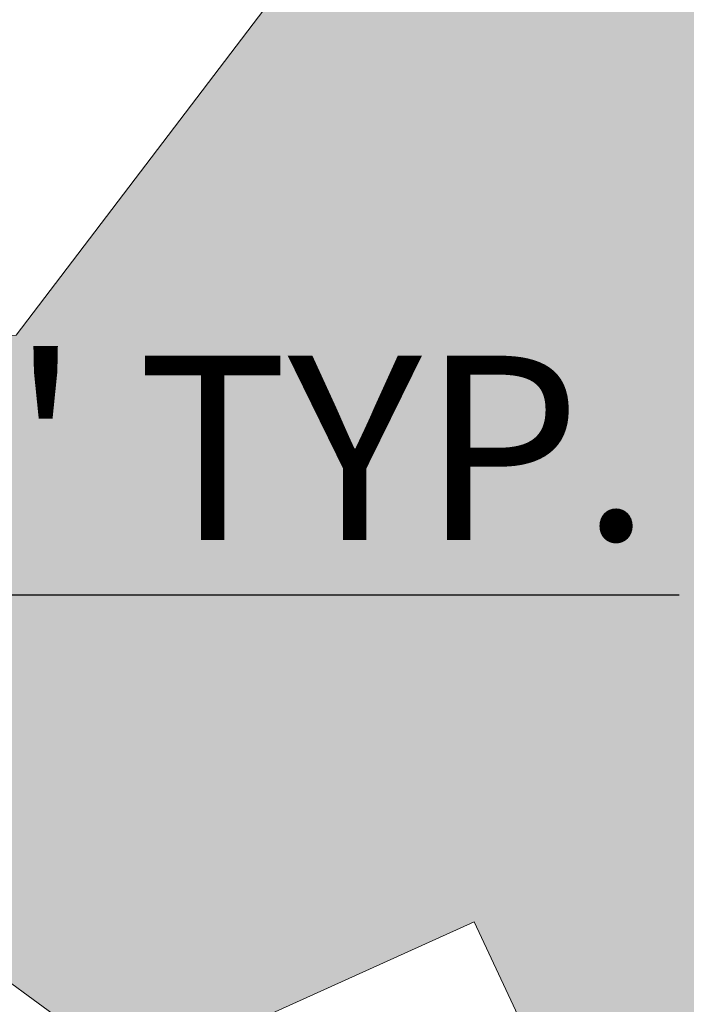
# Model space of a CAD drawing. Units: inches. Extents: x 2091 to 2899, y 967 to 2217.
# Tile 254 of 256: x 2232 to 2246, y 1131 to 1153. Entities that reach past the tile are written whole.
import ezdxf

# ---------------------------------------------------------------- set-up
doc = ezdxf.new("R2010")
doc.units = ezdxf.units.IN
doc.layers.add('A-ANNO-DIMS', color=2, linetype='Continuous', lineweight=18)
doc.layers.add('L-PLNT-TREE', color=94, linetype='Continuous', lineweight=13)
doc.layers.add('A-WALL-PATT', color=141, linetype='Continuous', lineweight=13, true_color=0xadddf7)
doc.layers.add('L-PLNT-PATT', color=114, linetype='Continuous', lineweight=13, true_color=0x139b48)
doc.styles.get("Standard").update_dxf_attribs({"font": 'arial.ttf'})
doc.dimstyles.new('ISO-25', dxfattribs={"dimtxt": 4, "dimasz": 4, "dimexe": 1.25, "dimexo": 0.625, "dimtad": 1, "dimdec": 0, "dimlunit": 3, "dimtxsty": 'Standard', "dimcen": 2.5, "dimadec": 0, "dimazin": 0, "dimtfac": 1, "dimtdec": 0, "dimtmove": 0, "dimatfit": 3, "dimfxl": 1, "dimarcsym": 0})

# ---------------------------------------------------------------- blocks, each defined once
blk = doc.blocks.new('*U25')
blk.add_lwpolyline([(-1139.42368, 1783.79628), (-1216.11644, 1685.47796), (-1117.5111, 1601.2033), (-1051.7759, 1643.3419), (-1126.09884, 1521.20092), (-1072.10606, 1527.49758), (-1079.90386, 1416.93646), (-1259.93906, 1179.83508), (-1479.05978, 1165.78888), (-1577.66258, 1109.60662), (-1742.00312, 927.01364), (-1676.26538, 814.64658), (-1270.89408, 828.69278), (-1194.20386, 772.51052), (-1007.95074, 856.78518), (-876.4778, 575.87134), (-821.70016, 575.87134), (-569.71184, 884.87504)])
blk = doc.blocks.new('*D37')
at = {"layer": 'A-ANNO-DIMS', "color": 0, "lineweight": -2, "transparency": 16777216}
for p, q in [((2203.116, 1151.622), (2203.116, 1138.874)), ((2212.276, 1151.622), (2212.276, 1138.874)), ((2199.116, 1140.124), (2195.116, 1140.124)), ((2203.116, 1140.124), (2212.276, 1140.124)), ((2216.276, 1140.124), (2245.908, 1140.124))]:
    blk.add_line(p, q, dxfattribs=at)
at = {"layer": 'A-ANNO-DIMS', "color": 0, "transparency": 16777216}
for points in [[(2199.116, 1140.79), (2199.116, 1139.457), (2203.116, 1140.124)], [(2216.276, 1140.79), (2216.276, 1139.457), (2212.276, 1140.124)]]:
    blk.add_solid(points, dxfattribs=at)
at = {"layer": 'Defpoints', "color": 0, "transparency": 16777216}
for p in [(2203.116, 1152.247), (2212.276, 1152.247), (2212.276, 1140.124)]:
    blk.add_point(p, dxfattribs=at)
at = {"layer": 'A-ANNO-DIMS', "color": 0, "transparency": 16777216, "insert": (2233.092, 1142.791), "char_height": 4, "attachment_point": 5}
blk.add_mtext('0\'-9" TYP.', dxfattribs=at)
blk = doc.blocks.new('*D71')
at = {"layer": 'A-ANNO-DIMS', "color": 0, "lineweight": -2, "transparency": 16777216}
for p, q in [((2212.144, 1351.294), (2212.144, 969.464)), ((2452.144, 1351.294), (2452.144, 969.464)), ((2216.144, 970.714), (2448.144, 970.714))]:
    blk.add_line(p, q, dxfattribs=at)
at = {"layer": 'A-ANNO-DIMS', "color": 0, "transparency": 16777216}
for points in [[(2216.144, 971.381), (2216.144, 970.048), (2212.144, 970.714)], [(2448.144, 971.381), (2448.144, 970.048), (2452.144, 970.714)]]:
    blk.add_solid(points, dxfattribs=at)
at = {"layer": 'Defpoints', "color": 0, "transparency": 16777216}
for p in [(2212.144, 1351.919), (2452.144, 1351.919), (2452.144, 970.714)]:
    blk.add_point(p, dxfattribs=at)
at = {"layer": 'A-ANNO-DIMS', "color": 0, "transparency": 16777216, "insert": (2332.144, 973.382), "char_height": 4, "attachment_point": 5}
blk.add_mtext('20\'-0"', dxfattribs=at)

msp = doc.modelspace()

# ---------------------------------------------------------------- hatches: boundary and pattern name
at = {"layer": 'A-WALL-PATT'}
h = msp.add_hatch(color=256, dxfattribs=at)
h.dxf.hatch_style = 1
h.paths.add_polyline_path([(2803.144, 2050.919), (2203.144, 2050.919), (2203.144, 1090.919), (2803.144, 1090.919)])
h.paths.add_polyline_path([(2635.799, 1147.54), (2674.524, 1147.54, 0.376086), (2678.53, 1152.88), (2678.53, 1159.556, 0.333335), (2674.524, 1163.562), (2674.524, 1163.562), (2674.524, 1192.934), (2635.806, 1192.934), (2597.088, 1192.934), (2597.088, 1163.562, 0.333335), (2593.082, 1159.556), (2593.082, 1152.88, 0.376086), (2597.088, 1147.54)], flags=0)
h.paths.add_polyline_path([(2436.01, 1278.241, 0.000483), (2435.953, 1278.215, -0.001328), (2435.936, 1278.112, -0.001711), (2436.116, 1278.041, 0.002185)], flags=0)
h.paths.add_polyline_path([(2794.144, 1143.419), (2794.144, 1347.419), (2543.37, 1347.419), (2543.37, 1351.919), (2794.144, 1351.919), (2794.144, 1392.714), (2793.947, 1392.714), (2793.947, 1473.537), (2794.144, 1473.537), (2794.144, 1531.919), (2650.144, 1531.919), (2650.144, 1536.419), (2794.144, 1536.419), (2794.144, 1692.419), (2609.376, 1692.419), (2609.376, 1644.419), (2604.876, 1644.419), (2604.876, 1744.919), (2609.376, 1744.919), (2609.376, 1696.919), (2794.144, 1696.919), (2794.144, 1780.919), (2609.644, 1780.919), (2493.876, 1780.919), (2493.876, 1785.419), (2609.644, 1785.419), (2794.144, 1785.419), (2794.144, 1847.939), (2793.951, 1847.939), (2793.951, 1928.762), (2794.144, 1928.762), (2794.144, 1941.419), (2614.144, 1941.419), (2614.144, 1821.419), (2609.644, 1821.419), (2609.644, 1941.419), (2392.144, 1941.419), (2392.144, 1819.919), (2387.644, 1819.919), (2387.644, 1941.419), (2212.144, 1941.419), (2212.144, 1783.919), (2392.144, 1783.919), (2392.144, 1780.919), (2212.144, 1780.919), (2212.144, 1629.419), (2387.644, 1629.419), (2387.644, 1744.919), (2392.144, 1744.919), (2392.144, 1627.919), (2317.144, 1627.919), (2317.144, 1551.419), (2317.144, 1536.419), (2459.384, 1536.419), (2459.384, 1602.396), (2463.884, 1602.396), (2463.884, 1531.919), (2456.644, 1531.919), (2456.644, 1529.919), (2452.144, 1529.919), (2452.144, 1531.919), (2312.644, 1531.919), (2312.644, 1551.419), (2306.144, 1551.419), (2306.144, 1555.919), (2308.144, 1555.919), (2308.144, 1551.419), (2312.644, 1551.419), (2312.644, 1627.919), (2212.144, 1627.919), (2212.144, 1555.919), (2270.144, 1555.919), (2270.144, 1551.419), (2212.144, 1551.419), (2212.144, 1351.919), (2272.144, 1351.919), (2272.144, 1347.419), (2212.144, 1347.419), (2212.144, 1275.419), (2308.144, 1275.419), (2308.144, 1351.919), (2452.144, 1351.919), (2452.144, 1493.919), (2456.644, 1493.919), (2456.644, 1347.419), (2312.644, 1347.419), (2312.644, 1270.919), (2212.144, 1270.919), (2212.144, 1099.919), (2281.238, 1099.919), (2282.871, 1110.914), (2282.008, 1116.997), (2278.558, 1121.42), (2268.206, 1128.056), (2272.088, 1128.056), (2273.813, 1131.927), (2279.42, 1134.692), (2285.028, 1135.245), (2287.616, 1137.457), (2288.047, 1138.01), (2289.341, 1140.775), (2291.067, 1139.669), (2292.361, 1135.245), (2295.38, 1136.904), (2296.243, 1135.798), (2297.105, 1133.033), (2300.125, 1138.01), (2303.144, 1138.01), (2304.438, 1135.798), (2303.144, 1133.586), (2306.595, 1134.692), (2307.889, 1133.033), (2310.908, 1135.245), (2313.927, 1134.139), (2315.627, 1132.427), (2308.32, 1117.55), (2290.204, 1109.808), (2288.91, 1103.172), (2289.272, 1099.919), (2434.918, 1099.919), (2431.593, 1124.788), (2429.93, 1169.553), (2430.927, 1240.52), (2435.659, 1238.186), (2437.135, 1196.554), (2438.798, 1143.973), (2442.678, 1111.998), (2446.558, 1099.919), (2794.144, 1099.919), (2794.144, 1138.919), (2548.032, 1138.919), (2548.032, 1143.419), (2548.032, 1148.819), (2546.668, 1148.032), (2528.686, 1179.179, 0.256256), (2512.032, 1148.819), (2512.032, 1143.419), (2512.032, 1138.919), (2507.532, 1138.919), (2507.532, 1143.419), (2507.532, 1148.819, 0.256256), (2490.879, 1179.179), (2472.896, 1148.032), (2471.532, 1148.819), (2471.532, 1143.419), (2467.032, 1143.419), (2467.032, 1269.946, 0.039061), (2460.91, 1273.58), (2467.032, 1273.58), (2467.032, 1286.325, 0.014511), (2465.216, 1286.762), (2467.032, 1287.053), (2467.032, 1323.419), (2471.532, 1323.419), (2471.532, 1148.819), (2489.532, 1179.996), (2490.896, 1179.208), (2490.879, 1179.179, -0.256256), (2507.532, 1148.819), (2507.532, 1143.419), (2512.032, 1143.419), (2512.032, 1148.819, -0.256256), (2528.686, 1179.179), (2528.668, 1179.208), (2530.032, 1179.996), (2548.032, 1148.819), (2548.032, 1143.419)], flags=16)
h.paths.add_polyline_path([(2607.769, 1200.945), (2607.769, 1265.031), (2597.088, 1281.052), (2619.785, 1281.052), (2627.795, 1337.127), (2635.799, 1337.127), (2643.817, 1337.127), (2651.827, 1281.052), (2674.524, 1281.052), (2663.843, 1265.031), (2663.843, 1200.945), (2635.806, 1200.945)], flags=0)
edge = h.paths.add_edge_path(flags=0)
edge.add_ellipse((13303.896, 1272.999), major_axis=(-10595.313, 0), ratio=0.84230387, start_angle=0.6282372, end_angle=0.6465541, ccw=False)
edge.add_ellipse((2711.7, 1156.853), major_axis=(2.22, 0), ratio=0.842304, start_angle=111.5352, end_angle=180.6282, ccw=False)
edge.add_ellipse((13303.156, 1272.999), major_axis=(-10593.026, 0), ratio=0.84230387, start_angle=0.5282715, end_angle=0.6465541, ccw=False)
edge.add_line((2710.765, 1175.333), (2710.13, 1175.333))
edge.add_ellipse((2710.13, 1176.58), major_axis=(1.48, 0), ratio=0.842304, start_angle=180, end_angle=270, ccw=False)
edge.add_line((2708.65, 1176.58), (2708.65, 1200.783))
edge.add_ellipse((2710.13, 1200.783), major_axis=(1.48, 0), ratio=0.842304, start_angle=90, end_angle=180, ccw=False)
edge.add_line((2710.13, 1202.029), (2710.465, 1202.029))
edge.add_ellipse((13303.156, 1272.999), major_axis=(-10593.026, 0), ratio=0.84230387, start_angle=-0.0902291, end_angle=0.3838668, ccw=False)
edge.add_ellipse((2710.13, 1290.927), major_axis=(-1.48, 0), ratio=0.842304, start_angle=0, end_angle=90, ccw=False)
edge.add_line((2708.65, 1290.927), (2708.65, 1315.13))
edge.add_ellipse((2710.13, 1315.13), major_axis=(-1.48, 0), ratio=0.842304, start_angle=-90, end_angle=0, ccw=False)
edge.add_line((2710.13, 1316.377), (2710.706, 1316.377))
edge.add_ellipse((3238.402, 1296.29), major_axis=(528.234, 0), ratio=0.8423039, start_angle=176.34957, end_angle=177.82005, ccw=False)
edge.add_ellipse((2775.063, 1071.451), major_axis=(313.308, 0), ratio=0.8423039, start_angle=102.12597, end_angle=103.78053, ccw=False)
edge.add_ellipse((2775.063, 1078.306), major_axis=(-305.303, 0), ratio=0.8423039, start_angle=-79.79046, end_angle=-77.55537, ccw=False)
edge.add_ellipse((2695.142, 1541.975), major_axis=(-250.96, 0), ratio=0.8423039, start_angle=99.25657, end_angle=102.55493)
edge.add_line((2741.41, 1334.214), (2747.133, 1337.378))
edge.add_ellipse((2747.539, 1336.857), major_axis=(-0.74, 0), ratio=0.842304, start_angle=270, end_angle=307.9331, ccw=False)
edge.add_ellipse((2747.539, 1336.857), major_axis=(-0.74, 0), ratio=0.842304, start_angle=232.0669, end_angle=270, ccw=False)
edge.add_line((2747.945, 1337.378), (2753.667, 1334.214))
edge.add_ellipse((2799.935, 1541.975), major_axis=(250.96, 0), ratio=0.8423039, start_angle=257.44507, end_angle=260.74343)
edge.add_ellipse((2720.014, 1078.306), major_axis=(305.303, 0), ratio=0.8423039, start_angle=77.55537, end_angle=79.79046, ccw=False)
edge.add_ellipse((2720.014, 1071.451), major_axis=(-313.308, 0), ratio=0.8423039, start_angle=256.21947, end_angle=257.87403, ccw=False)
edge.add_ellipse((2256.676, 1296.29), major_axis=(-528.234, 0), ratio=0.8423039, start_angle=182.17995, end_angle=183.65043, ccw=False)
edge.add_line((2784.371, 1316.377), (2784.947, 1316.377))
edge.add_ellipse((2784.947, 1315.13), major_axis=(1.48, 0), ratio=0.842304, start_angle=0, end_angle=90, ccw=False)
edge.add_line((2786.427, 1315.13), (2786.427, 1290.927))
edge.add_ellipse((2784.947, 1290.927), major_axis=(1.48, 0), ratio=0.842304, start_angle=270, end_angle=360, ccw=False)
edge.add_ellipse((-7808.079, 1272.999), major_axis=(10593.026, 0), ratio=0.84230387, start_angle=-0.3838668, end_angle=0.0902291, ccw=False)
edge.add_line((2784.612, 1202.029), (2784.947, 1202.029))
edge.add_ellipse((2784.947, 1200.783), major_axis=(1.48, 0), ratio=0.842304, start_angle=0, end_angle=90, ccw=False)
edge.add_line((2786.427, 1200.783), (2786.427, 1176.58))
edge.add_ellipse((2784.947, 1176.58), major_axis=(-1.48, 0), ratio=0.842304, start_angle=90, end_angle=180, ccw=False)
edge.add_line((2784.947, 1175.333), (2784.313, 1175.333))
edge.add_ellipse((-7808.079, 1272.999), major_axis=(10593.026, 0), ratio=0.84230387, start_angle=-0.6186432, end_angle=-0.5282715, ccw=False)
edge.add_ellipse((2783.377, 1156.853), major_axis=(-2.22, 0), ratio=0.842304, start_angle=179.3718, end_angle=248.4648, ccw=False)
edge.add_ellipse((-7808.819, 1272.999), major_axis=(-10595.313, 0), ratio=0.842303866, start_angle=179.3534459, end_angle=179.3717628, ccw=False)
edge.add_ellipse((2780.297, 1153.501), major_axis=(-5.246, 0), ratio=0.842304, start_angle=90, end_angle=179.3534, ccw=False)
edge.add_line((2780.297, 1149.082), (2714.78, 1149.082))
edge.add_ellipse((2714.78, 1153.501), major_axis=(5.246, 0), ratio=0.842304, start_angle=180.6466, end_angle=270, ccw=False)
edge = h.paths.add_edge_path(flags=0)
edge.add_line((2718.187, 1151.008), (2718.187, 1170.472))
edge.add_ellipse((2721.147, 1170.472), major_axis=(-2.96, 0), ratio=0.842304, start_angle=-90, end_angle=0, ccw=False)
edge.add_line((2721.147, 1172.965), (2773.93, 1172.965))
edge.add_ellipse((2773.93, 1170.472), major_axis=(-2.96, 0), ratio=0.842304, start_angle=180, end_angle=270, ccw=False)
edge.add_line((2776.89, 1170.472), (2776.89, 1151.008))
edge.add_line((2776.89, 1151.008), (2718.187, 1151.008))
edge = h.paths.add_edge_path(flags=0)
edge.add_line((2718.187, 1180.234), (2718.187, 1199.058))
edge.add_ellipse((2747.539, 1320.399), major_axis=(147.018, 0), ratio=0.8423039, start_angle=256.40187, end_angle=283.59813)
edge.add_line((2776.89, 1199.058), (2776.89, 1180.234))
edge.add_ellipse((2747.539, 1301.575), major_axis=(147.018, 0), ratio=0.8423039, start_angle=256.40187, end_angle=283.59813, ccw=False)
edge = h.paths.add_edge_path(flags=0)
edge.add_ellipse((13303.156, 1272.999), major_axis=(-10591.546, 0), ratio=0.84230387, start_angle=0.0555943, end_angle=0.3777642, ccw=False)
edge.add_line((2711.617, 1262.722), (2715.667, 1249.495))
edge.add_ellipse((6413.892, 1241.692), major_axis=(-3698.236, 0), ratio=0.84230387, start_angle=-0.120897, end_angle=0.364076)
edge.add_line((2715.761, 1218.192), (2711.934, 1203.167))
edge = h.paths.add_edge_path(flags=0)
edge.add_line((2718.187, 1251.075), (2716.002, 1267.45))
edge.add_ellipse((2742.151, 1202.19), major_axis=(81.773, 0), ratio=0.842304, start_angle=94.27742, end_angle=111.83495, ccw=False)
edge.add_line((2737.01, 1270.931), (2758.067, 1270.931))
edge.add_ellipse((2752.926, 1202.19), major_axis=(81.773, 0), ratio=0.842304, start_angle=68.16505, end_angle=85.72258, ccw=False)
edge.add_line((2779.075, 1267.45), (2776.89, 1251.075))
edge.add_ellipse((2750.338, 1187.885), major_axis=(79.58, 0), ratio=0.842304, start_angle=67.20809, end_angle=85.12993)
edge.add_line((2756.035, 1254.744), (2739.043, 1254.744))
edge.add_ellipse((2744.739, 1187.885), major_axis=(79.58, 0), ratio=0.842304, start_angle=94.87007, end_angle=112.79191)
edge = h.paths.add_edge_path(flags=0)
edge.add_line((2783.143, 1203.167), (2779.316, 1218.192))
edge.add_ellipse((-918.815, 1241.692), major_axis=(3698.236, 0), ratio=0.84230387, start_angle=-0.364076, end_angle=0.120897)
edge.add_line((2779.41, 1249.495), (2783.46, 1262.722))
edge.add_ellipse((-7808.079, 1272.999), major_axis=(-10591.546, 0), ratio=0.84230387, start_angle=179.6222358, end_angle=179.9444057, ccw=False)
edge = h.paths.add_edge_path(flags=0)
edge.add_ellipse((2734.201, 1286.69), major_axis=(-0.357, 6.34), ratio=0.603834, start_angle=89.002, end_angle=253.6574, ccw=False)
edge.add_line((2730.369, 1286.542), (2730.369, 1301.352))
edge.add_line((2730.369, 1301.352), (2735.913, 1305.215))
edge.add_ellipse((2736.385, 1304.735), major_axis=(0.74, 0), ratio=0.842304, start_angle=90, end_angle=134.4802, ccw=False)
edge.add_line((2736.385, 1305.358), (2738.033, 1305.358))
edge.add_line((2738.033, 1305.358), (2738.033, 1307.708))
edge.add_ellipse((2794.202, 1307.708), major_axis=(56.169, 0), ratio=0.842304, start_angle=150.5614, end_angle=180, ccw=False)
edge.add_ellipse((2700.876, 1307.708), major_axis=(-56.169, 0), ratio=0.842304, start_angle=180, end_angle=209.4386, ccw=False)
edge.add_line((2757.044, 1307.708), (2757.044, 1305.358))
edge.add_line((2757.044, 1305.358), (2758.692, 1305.358))
edge.add_ellipse((2758.692, 1304.735), major_axis=(-0.74, 0), ratio=0.842304, start_angle=225.5198, end_angle=270, ccw=False)
edge.add_line((2759.164, 1305.215), (2764.708, 1301.352))
edge.add_line((2764.708, 1301.352), (2764.708, 1286.542))
edge.add_ellipse((2760.876, 1286.69), major_axis=(0.357, 6.34), ratio=0.603834, start_angle=106.3426, end_angle=270.998, ccw=False)
edge.add_line((2757.044, 1285.797), (2757.044, 1307.708))
edge.add_ellipse((2700.876, 1307.708), major_axis=(-56.169, 0), ratio=0.842304, start_angle=180, end_angle=209.4386)
edge.add_ellipse((2794.202, 1307.708), major_axis=(56.169, 0), ratio=0.842304, start_angle=150.5614, end_angle=180)
edge.add_line((2738.033, 1307.708), (2738.033, 1285.797))
h.paths.add_polyline_path([(2417.812, 1104.45), (2413.492, 1102.53), (2410.612, 1103.97), (2409.172, 1106.37), (2407.252, 1107.33), (2406.292, 1109.73), (2405.332, 1114.05), (2405.332, 1117.89), (2406.292, 1120.13), (2407.252, 1119.81), (2408.848, 1118.328), (2410.174, 1119.424), (2410.211, 1120.406), (2411.041, 1121.419), (2410.699, 1119.859), (2410.174, 1119.424), (2410.088, 1117.176), (2411.133, 1116.206), (2413.972, 1119.33), (2416.852, 1120.77), (2416.87, 1120.799), (2417.035, 1119.405), (2417.896, 1118.143), (2418.292, 1118.37), (2419.544, 1120.039), (2419.361, 1118.387), (2419.032, 1119.356), (2418.399, 1118.512), (2419.252, 1114.53), (2418.794, 1107.199)], flags=0)
h.paths.add_polyline_path([(2508.87, 1347.419), (2508.37, 1347.419), (2508.37, 1351.919), (2508.87, 1351.919)], flags=0)
h.paths.add_polyline_path([(2473.37, 1347.419), (2472.37, 1347.419), (2467.87, 1347.419), (2467.87, 1455.419), (2472.37, 1455.419), (2472.37, 1352.419), (2473.37, 1352.419)], flags=0)
h.paths.add_polyline_path([(2352.106, 1217.446), (2349.226, 1218.886), (2347.786, 1221.286), (2345.866, 1222.246), (2344.906, 1224.646), (2343.946, 1228.966), (2343.946, 1232.806), (2344.906, 1235.046), (2345.866, 1234.726), (2347.462, 1233.244), (2348.788, 1234.341), (2348.825, 1235.322), (2349.655, 1236.336), (2349.313, 1234.775), (2348.788, 1234.341), (2348.702, 1232.093), (2349.747, 1231.123), (2352.586, 1234.246), (2355.466, 1235.686), (2355.484, 1235.715), (2355.649, 1234.322), (2356.51, 1233.06), (2356.906, 1233.286), (2358.158, 1234.956), (2357.975, 1233.304), (2357.646, 1234.273), (2357.013, 1233.428), (2357.866, 1229.446), (2357.408, 1222.115), (2356.426, 1219.366)], flags=0)
h.paths.add_polyline_path([(2348.297, 1112.224), (2347.014, 1112.31), (2345.53, 1114.127), (2345.732, 1115.858), (2346.812, 1116.982), (2346.812, 1114.646), (2345.867, 1114.214), (2346.88, 1114.3)], flags=0)
h.paths.add_polyline_path([(2347.014, 1110.926), (2346.272, 1110.493), (2346.61, 1111.186)], flags=0)
h.paths.add_polyline_path([(2345.867, 1118.194), (2345.53, 1117.329), (2343.708, 1118.021), (2344.383, 1118.626)], flags=0)
h.paths.add_polyline_path([(2346.677, 1109.282), (2346.07, 1108.071), (2345.867, 1110.061)], flags=0)
h.paths.add_polyline_path([(2345.057, 1119.751), (2343.64, 1119.751), (2343.978, 1121.135)], flags=0)
h.paths.add_polyline_path([(2345.26, 1116.55), (2345.125, 1115.858), (2344.922, 1115.685), (2344.72, 1116.377)], flags=0)
h.paths.add_polyline_path([(2345.665, 1112.31), (2345.462, 1111.532), (2344.045, 1111.964), (2344.652, 1112.57)], flags=0)
h.paths.add_polyline_path([(2345.192, 1113.349), (2344.45, 1113.868), (2344.72, 1114.387)], flags=0)
h.paths.add_polyline_path([(2344.652, 1116.809), (2344.18, 1115.685), (2344.652, 1115.339), (2343.91, 1114.906), (2343.033, 1115.944), (2343.64, 1116.463)], flags=0)
h.paths.add_polyline_path([(2345.867, 1106.686), (2344.99, 1105.562), (2344.517, 1106.6)], flags=0)
h.paths.add_polyline_path([(2344.855, 1110.061), (2344.517, 1109.282), (2344.113, 1109.715)], flags=0)
h.paths.add_polyline_path([(2344.045, 1113.522), (2343.438, 1113.089), (2342.763, 1113.954)], flags=0)
h.paths.add_polyline_path([(2344.315, 1111.012), (2342.965, 1110.32), (2342.965, 1111.099)], flags=0)
h.paths.add_polyline_path([(2345.125, 1104.697), (2344.585, 1103.745), (2344.45, 1104.264)], flags=0)
h.paths.add_polyline_path([(2342.83, 1121.222), (2341.75, 1120.53), (2340.536, 1121.049), (2340.131, 1121.828), (2340.671, 1122.952), (2341.143, 1121.828), (2341.615, 1122.001)], flags=0)
h.paths.add_polyline_path([(2342.965, 1119.751), (2343.033, 1118.453), (2342.088, 1118.021), (2342.02, 1119.491)], flags=0)
h.paths.add_polyline_path([(2342.695, 1116.896), (2341.953, 1116.636), (2342.02, 1117.329)], flags=0)
h.paths.add_polyline_path([(2343.033, 1112.224), (2342.02, 1111.791), (2341.548, 1112.224), (2342.358, 1113.349)], flags=0)
h.paths.add_polyline_path([(2343.775, 1104.437), (2342.628, 1102.88), (2342.695, 1104.61), (2343.438, 1105.129)], flags=0)
h.paths.add_polyline_path([(2342.02, 1115.079), (2340.806, 1115.512), (2340.941, 1116.377)], flags=0)
h.paths.add_polyline_path([(2341.481, 1120.097), (2341.481, 1119.405), (2341.076, 1119.578), (2341.143, 1120.097)], flags=0)
h.paths.add_polyline_path([(2341.818, 1114.473), (2340.941, 1113.089), (2340.806, 1114.56)], flags=0)
h.paths.add_polyline_path([(2341.143, 1118.54), (2340.941, 1116.982), (2339.051, 1117.675), (2339.051, 1118.626)], flags=0)
h.paths.add_polyline_path([(2342.695, 1101.668), (2341.953, 1101.841), (2342.56, 1102.361)], flags=0)
h.paths.add_polyline_path([(2340.333, 1119.665), (2338.444, 1119.578), (2337.904, 1120.357), (2339.658, 1120.616)], flags=0)
h.paths.add_polyline_path([(2340.333, 1115.339), (2340.063, 1113.695), (2339.388, 1115.339)], flags=0)
h.paths.add_polyline_path([(2341.818, 1103.831), (2341.548, 1102.88), (2341.143, 1103.658)], flags=0)
h.paths.add_polyline_path([(2339.051, 1122.866), (2337.296, 1121.828), (2337.094, 1123.125), (2337.769, 1123.818)], flags=0)
h.paths.add_polyline_path([(2339.118, 1121.741), (2338.848, 1121.222), (2338.174, 1121.049), (2338.376, 1121.568)], flags=0)
h.paths.add_polyline_path([(2339.186, 1119.319), (2338.646, 1118.713), (2338.241, 1118.107), (2338.241, 1118.886)], flags=0)
h.paths.add_polyline_path([(2341.143, 1101.928), (2340.603, 1101.236), (2340.063, 1101.841), (2340.603, 1102.361)], flags=0)
h.paths.add_polyline_path([(2337.634, 1117.761), (2336.621, 1118.28), (2337.296, 1118.972)], flags=0)
h.paths.add_polyline_path([(2336.824, 1119.578), (2334.799, 1118.972), (2335.204, 1120.357), (2336.554, 1120.876)], flags=0)
h.paths.add_polyline_path([(2339.118, 1100.457), (2337.364, 1100.543), (2336.756, 1101.236)], flags=0)
h.paths.add_polyline_path([(2336.351, 1122.433), (2336.014, 1121.914), (2334.934, 1122.433), (2334.529, 1123.471), (2335.744, 1122.779)], flags=0)
h.paths.add_polyline_path([(2334.732, 1120.876), (2334.259, 1120.357), (2334.057, 1120.789), (2334.597, 1121.308)], flags=0)
h.paths.add_polyline_path([(2334.462, 1122.174), (2332.572, 1121.308), (2331.357, 1122.174), (2332.1, 1122.866)], flags=0)
h.paths.add_polyline_path([(2334.259, 1118.54), (2333.382, 1118.453), (2333.652, 1119.319)], flags=0)
h.paths.add_polyline_path([(2335.542, 1102.274), (2334.192, 1102.62), (2335.272, 1103.312)], flags=0)
h.paths.add_polyline_path([(2332.707, 1119.665), (2331.695, 1120.443), (2332.505, 1120.789)], flags=0)
h.paths.add_polyline_path([(2334.732, 1101.149), (2333.517, 1101.582), (2333.989, 1101.755)], flags=0)
h.paths.add_polyline_path([(2332.64, 1116.636), (2331.087, 1116.29), (2331.965, 1118.194)], flags=0)
h.paths.add_polyline_path([(2330.75, 1121.568), (2330.277, 1120.27), (2328.523, 1119.319), (2328.995, 1121.049)], flags=0)
h.paths.add_polyline_path([(2330.75, 1118.626), (2330.008, 1117.502), (2329.873, 1118.021)], flags=0)
h.paths.add_polyline_path([(2332.1, 1102.361), (2330.547, 1102.014), (2331.695, 1102.966)], flags=0)
h.paths.add_polyline_path([(2329.535, 1113.608), (2329.063, 1112.31), (2328.59, 1113.349)], flags=0)
h.paths.add_polyline_path([(2328.388, 1117.848), (2327.51, 1116.55), (2327.173, 1117.761)], flags=0)
h.paths.add_polyline_path([(2329.738, 1106.513), (2329.535, 1105.302), (2328.253, 1106.081)], flags=0)
h.paths.add_polyline_path([(2328.658, 1114.387), (2328.05, 1114.127), (2328.32, 1114.906)], flags=0)
h.paths.add_polyline_path([(2328.32, 1112.224), (2327.106, 1112.137), (2326.701, 1112.656)], flags=0)
h.paths.add_polyline_path([(2326.903, 1115.252), (2326.701, 1114.127), (2325.216, 1113.608), (2326.093, 1115.339)], flags=0)
h.paths.add_polyline_path([(2326.633, 1108.33), (2326.093, 1107.379), (2325.891, 1108.503), (2326.498, 1109.109)], flags=0)
h.paths.add_polyline_path([(2615.144, 1531.919), (2609.644, 1531.919), (2609.644, 1620.419), (2614.144, 1620.419), (2614.144, 1536.419), (2615.144, 1536.419)], flags=0)
h.paths.add_polyline_path([(2545.144, 1563.419), (2464.144, 1563.419), (2464.144, 1632.419), (2509.144, 1632.419), (2509.144, 1627.919), (2509.144, 1603.919), (2468.644, 1603.919), (2468.644, 1567.919), (2540.644, 1567.919), (2540.644, 1591.919), (2545.144, 1591.919)], flags=0)
h.paths.add_polyline_path([(2388.969, 1549.986), (2357.434, 1549.986), (2357.434, 1623.361), (2399.363, 1623.361), (2435.689, 1623.361), (2435.593, 1602.559), (2435.593, 1602.396), (2388.969, 1602.396)], flags=0)
h.paths.add_polyline_path([(2388.881, 1555.809), (2374.904, 1555.809), (2374.904, 1600.572), (2374.904, 1615.458), (2406.351, 1615.458), (2406.351, 1618.939), (2412.174, 1615.458), (2406.351, 1611.976), (2406.351, 1615.458), (2388.881, 1615.458)], flags=0)
h.paths.add_polyline_path([(2568.876, 1644.419), (2453.376, 1644.419), (2453.376, 1785.419), (2457.876, 1785.419), (2457.876, 1648.919), (2568.876, 1648.919)], flags=0)
h.paths.add_polyline_path([(2212.144, 1945.919), (2212.144, 2041.919), (2794.144, 2041.919), (2794.144, 1945.919)], flags=16)
h.paths.add_polyline_path([(2271.083, 1964.317), (2776.853, 1964.317), (2776.853, 2037.17), (2271.083, 2037.17)], flags=8)
h.paths.add_polyline_path([(2380.649, 1536.824), (2461.041, 1536.824), (2461.041, 1554.653), (2380.649, 1554.653)], flags=8)
h.paths.add_polyline_path([(2240.756, 1609.725), (2309.186, 1609.725), (2309.186, 1617.698), (2240.756, 1617.698)], flags=8)
h.paths.add_polyline_path([(2212.677, 1313.504), (2282.592, 1313.504), (2282.592, 1322.745), (2212.677, 1322.745)], flags=8)
h.paths.add_polyline_path([(2457.112, 1114.779), (2558.482, 1114.779), (2558.482, 1142.22), (2457.112, 1142.22)], flags=8)
h.paths.add_polyline_path([(2473.442, 1273.01), (2604.641, 1273.01), (2604.641, 1318.347), (2473.442, 1318.347)], flags=8)
h.paths.add_polyline_path([(2638.876, 1626.977), (2684.25, 1627.977), (2684.038, 1637.597), (2638.664, 1636.598)], flags=8)
h.paths.add_polyline_path([(2537.591, 1453.793), (2628.39, 1453.793), (2628.39, 1475.345), (2537.591, 1475.345)], flags=8)
h.paths.add_polyline_path([(2504.138, 1714.632), (2554.647, 1714.632), (2554.647, 1730.238), (2504.138, 1730.238)], flags=8)
h.paths.add_polyline_path([(2487.501, 1575.652), (2535.097, 1575.652), (2535.097, 1598.378), (2487.501, 1598.378)], flags=8)
h.paths.add_polyline_path([(2709.099, 1735.71), (2740.017, 1735.71), (2740.017, 1749.938), (2709.099, 1749.938)], flags=8)
h.paths.add_polyline_path([(2442.438, 1792.172), (2564.729, 1792.172), (2564.729, 1842), (2442.438, 1842)], flags=8)
h.paths.add_polyline_path([(2655.816, 1809.644), (2789.52, 1806.694), (2790.085, 1832.292), (2656.381, 1835.242)], flags=8)
h.paths.add_polyline_path([(2234.843, 1797.72), (2368.593, 1794.769), (2369.161, 1820.504), (2235.411, 1823.455)], flags=8)
h.paths.add_polyline_path([(2245.138, 1644.006), (2398.428, 1640.624), (2398.995, 1666.325), (2245.706, 1669.707)], flags=8)
h.paths.add_polyline_path([(2306.143, 1431.169), (2413.768, 1428.794), (2414.333, 1454.392), (2306.708, 1456.766)], flags=8)
h.paths.add_polyline_path([(2306.835, 1458.233), (2393.38, 1456.323), (2393.933, 1481.354), (2307.387, 1483.264)], flags=8)
at = {"layer": 'L-PLNT-PATT'}
h = msp.add_hatch(color=256, dxfattribs=at)
h.dxf.hatch_style = 1
h.paths.add_polyline_path([(2333.338, 1165.659), (2329.024, 1166.212), (2331.612, 1168.424), (2335.063, 1177.271), (2328.162, 1184.46), (2319.535, 1187.225), (2323.417, 1193.308), (2319.966, 1203.814), (2317.809, 1203.814), (2313.496, 1213.215), (2310.908, 1212.662), (2307.889, 1212.662), (2305.732, 1217.086), (2307.026, 1223.168), (2310.477, 1223.168), (2304.007, 1230.91), (2303.136, 1237.046), (2299.693, 1240.864), (2296.674, 1237.546), (2294.949, 1238.652), (2294.517, 1241.417), (2292.361, 1242.523), (2289.341, 1239.758), (2285.89, 1240.311), (2283.302, 1235.334), (2283.302, 1230.91), (2286.753, 1229.251), (2284.165, 1227.592), (2281.577, 1229.804), (2274.244, 1222.615), (2274.244, 1220.957), (2271.225, 1219.298), (2272.088, 1217.639), (2274.244, 1214.321), (2270.362, 1211.556), (2266.48, 1214.321), (2264.324, 1213.768), (2263.461, 1211.556), (2266.48, 1211.003), (2266.912, 1206.579), (2263.539, 1207.132), (2259.579, 1203.261), (2263.892, 1202.708), (2262.167, 1197.178), (2258.285, 1196.625), (2253.971, 1193.861), (2248.795, 1191.096), (2248.364, 1193.308), (2244.482, 1185.013), (2251.383, 1186.672), (2255.697, 1183.907), (2254.403, 1177.271), (2246.639, 1174.506), (2243.188, 1176.718), (2241.894, 1173.4), (2238.875, 1172.847), (2236.287, 1169.53), (2233.267, 1165.659), (2237.149, 1162.341), (2239.737, 1164), (2236.811, 1159.191), (2238.937, 1159.439), (2238.63, 1155.086), (2231.542, 1145.752), (2222.915, 1145.199), (2219.033, 1142.987), (2212.563, 1135.798), (2215.151, 1131.374), (2231.111, 1131.927), (2234.13, 1129.715), (2241.463, 1133.033), (2246.639, 1121.973), (2248.795, 1121.973), (2258.716, 1134.139), (2261.736, 1135.798), (2263.892, 1133.033), (2263.892, 1129.162), (2267.343, 1128.056), (2272.088, 1128.056), (2273.813, 1131.927), (2279.42, 1134.692), (2285.028, 1135.245), (2287.616, 1137.457), (2288.047, 1138.01), (2289.341, 1140.775), (2291.067, 1139.669), (2292.361, 1135.245), (2295.38, 1136.904), (2296.243, 1135.798), (2297.105, 1133.033), (2300.125, 1138.01), (2303.144, 1138.01), (2304.438, 1135.798), (2303.144, 1133.586), (2306.595, 1134.692), (2307.889, 1133.033), (2310.908, 1135.245), (2313.927, 1134.139), (2319.966, 1128.056), (2322.554, 1126.95), (2324.711, 1124.738), (2342.827, 1126.397), (2346.278, 1123.079), (2348.866, 1124.185), (2341.964, 1133.033), (2341.533, 1136.351), (2343.69, 1139.669), (2339.808, 1150.175), (2337.651, 1150.175)])
h.paths.add_polyline_path([(2339.658, 1120.616), (2337.904, 1120.357), (2338.444, 1119.578), (2340.333, 1119.665)])
h.paths.add_polyline_path([(2341.143, 1118.54), (2339.051, 1118.626), (2339.051, 1117.675), (2340.941, 1116.982)])
h.paths.add_polyline_path([(2336.554, 1120.876), (2335.204, 1120.357), (2334.799, 1118.972), (2336.824, 1119.578)])
h.paths.add_polyline_path([(2337.296, 1118.972), (2336.621, 1118.28), (2337.634, 1117.761)])
h.paths.add_polyline_path([(2338.646, 1118.713), (2339.186, 1119.319), (2338.241, 1118.886), (2338.241, 1118.107)])
h.paths.add_polyline_path([(2339.051, 1122.866), (2337.769, 1123.818), (2337.094, 1123.125), (2337.296, 1121.828)])
h.paths.add_polyline_path([(2341.615, 1122.001), (2341.143, 1121.828), (2340.671, 1122.952), (2340.131, 1121.828), (2340.536, 1121.049), (2341.75, 1120.53), (2342.83, 1121.222)])
h.paths.add_polyline_path([(2342.965, 1119.751), (2342.02, 1119.491), (2342.088, 1118.021), (2343.033, 1118.453)])
h.paths.add_polyline_path([(2345.867, 1118.194), (2344.383, 1118.626), (2343.708, 1118.021), (2345.53, 1117.329)])
h.paths.add_polyline_path([(2344.652, 1116.809), (2343.64, 1116.463), (2343.033, 1115.944), (2343.91, 1114.906), (2344.652, 1115.339), (2344.18, 1115.685)])
h.paths.add_polyline_path([(2346.812, 1116.982), (2345.732, 1115.858), (2345.53, 1114.127), (2347.014, 1112.31), (2348.297, 1112.224), (2346.88, 1114.3), (2345.867, 1114.214), (2346.812, 1114.646)])
h.paths.add_polyline_path([(2345.26, 1116.55), (2344.72, 1116.377), (2344.922, 1115.685), (2345.125, 1115.858)])
h.paths.add_polyline_path([(2342.695, 1116.896), (2342.02, 1117.329), (2341.953, 1116.636)])
h.paths.add_polyline_path([(2341.481, 1120.097), (2341.143, 1120.097), (2341.076, 1119.578), (2341.481, 1119.405)])
h.paths.add_polyline_path([(2343.978, 1121.135), (2343.64, 1119.751), (2345.057, 1119.751)])
h.paths.add_polyline_path([(2339.118, 1121.741), (2338.376, 1121.568), (2338.174, 1121.049), (2338.848, 1121.222)])
h.paths.add_polyline_path([(2336.351, 1122.433), (2335.744, 1122.779), (2334.529, 1123.471), (2334.934, 1122.433), (2336.014, 1121.914)])
h.paths.add_polyline_path([(2334.462, 1122.174), (2332.1, 1122.866), (2331.357, 1122.174), (2332.572, 1121.308)])
h.paths.add_polyline_path([(2334.597, 1121.308), (2334.057, 1120.789), (2334.259, 1120.357), (2334.732, 1120.876)])
h.paths.add_polyline_path([(2332.505, 1120.789), (2331.695, 1120.443), (2332.707, 1119.665)])
h.paths.add_polyline_path([(2333.652, 1119.319), (2333.382, 1118.453), (2334.259, 1118.54)])
h.paths.add_polyline_path([(2331.965, 1118.194), (2331.087, 1116.29), (2332.64, 1116.636)])
h.paths.add_polyline_path([(2330.75, 1121.568), (2328.995, 1121.049), (2328.523, 1119.319), (2330.277, 1120.27)])
h.paths.add_polyline_path([(2330.75, 1118.626), (2329.873, 1118.021), (2330.008, 1117.502)])
h.paths.add_polyline_path([(2328.388, 1117.848), (2327.173, 1117.761), (2327.51, 1116.55)])
h.paths.add_polyline_path([(2326.903, 1115.252), (2326.093, 1115.339), (2325.216, 1113.608), (2326.701, 1114.127)])
h.paths.add_polyline_path([(2328.658, 1114.387), (2328.32, 1114.906), (2328.05, 1114.127)])
h.paths.add_polyline_path([(2326.701, 1112.656), (2327.106, 1112.137), (2328.32, 1112.224)])
h.paths.add_polyline_path([(2329.535, 1113.608), (2328.59, 1113.349), (2329.063, 1112.31)])
h.paths.add_polyline_path([(2340.333, 1115.339), (2339.388, 1115.339), (2340.063, 1113.695)])
h.paths.add_polyline_path([(2340.941, 1116.377), (2340.806, 1115.512), (2342.02, 1115.079)])
h.paths.add_polyline_path([(2341.818, 1114.473), (2340.806, 1114.56), (2340.941, 1113.089)])
h.paths.add_polyline_path([(2343.033, 1112.224), (2342.358, 1113.349), (2341.548, 1112.224), (2342.02, 1111.791)])
h.paths.add_polyline_path([(2342.763, 1113.954), (2343.438, 1113.089), (2344.045, 1113.522)])
h.paths.add_polyline_path([(2344.72, 1114.387), (2344.45, 1113.868), (2345.192, 1113.349)])
h.paths.add_polyline_path([(2345.665, 1112.31), (2344.652, 1112.57), (2344.045, 1111.964), (2345.462, 1111.532)])
h.paths.add_polyline_path([(2344.315, 1111.012), (2342.965, 1111.099), (2342.965, 1110.32)])
h.paths.add_polyline_path([(2344.855, 1110.061), (2344.113, 1109.715), (2344.517, 1109.282)])
h.paths.add_polyline_path([(2346.677, 1109.282), (2345.867, 1110.061), (2346.07, 1108.071)])
h.paths.add_polyline_path([(2347.014, 1110.926), (2346.61, 1111.186), (2346.272, 1110.493)])
h.paths.add_polyline_path([(2345.867, 1106.686), (2344.517, 1106.6), (2344.99, 1105.562)])
h.paths.add_polyline_path([(2345.125, 1104.697), (2344.45, 1104.264), (2344.585, 1103.745)])
h.paths.add_polyline_path([(2343.775, 1104.437), (2343.438, 1105.129), (2342.695, 1104.61), (2342.628, 1102.88)])
h.paths.add_polyline_path([(2341.818, 1103.831), (2341.143, 1103.658), (2341.548, 1102.88)])
h.paths.add_polyline_path([(2342.56, 1102.361), (2341.953, 1101.841), (2342.695, 1101.668)])
h.paths.add_polyline_path([(2341.143, 1101.928), (2340.603, 1102.361), (2340.063, 1101.841), (2340.603, 1101.236)])
h.paths.add_polyline_path([(2336.756, 1101.236), (2337.364, 1100.543), (2339.118, 1100.457)])
h.paths.add_polyline_path([(2335.272, 1103.312), (2334.192, 1102.62), (2335.542, 1102.274)])
h.paths.add_polyline_path([(2333.989, 1101.755), (2333.517, 1101.582), (2334.732, 1101.149)])
h.paths.add_polyline_path([(2331.695, 1102.966), (2330.547, 1102.014), (2332.1, 1102.361)])
h.paths.add_polyline_path([(2329.738, 1106.513), (2328.253, 1106.081), (2329.535, 1105.302)])
h.paths.add_polyline_path([(2326.633, 1108.33), (2326.498, 1109.109), (2325.891, 1108.503), (2326.093, 1107.379)])
h.paths.add_polyline_path([(2240.596, 1257.814), (2239.584, 1257.468), (2238.977, 1256.949), (2239.854, 1255.911), (2240.596, 1256.344), (2240.124, 1256.69)])
h.paths.add_polyline_path([(2241.811, 1259.199), (2240.327, 1259.631), (2239.652, 1259.026), (2241.474, 1258.334)])
h.paths.add_polyline_path([(2242.756, 1257.987), (2241.676, 1256.863), (2241.474, 1255.132), (2242.958, 1253.315), (2244.241, 1253.229), (2242.824, 1255.305), (2241.811, 1255.219), (2242.756, 1255.651)])
h.paths.add_polyline_path([(2241.609, 1253.315), (2240.596, 1253.575), (2239.989, 1252.969), (2241.406, 1252.537)])
h.paths.add_polyline_path([(2240.664, 1255.392), (2240.394, 1254.873), (2241.136, 1254.354)])
h.paths.add_polyline_path([(2242.958, 1251.931), (2242.554, 1252.191), (2242.216, 1251.498)])
h.paths.add_polyline_path([(2240.259, 1252.017), (2238.909, 1252.104), (2238.909, 1251.325)])
h.paths.add_polyline_path([(2238.302, 1254.354), (2237.492, 1253.229), (2237.964, 1252.796), (2238.977, 1253.229)])
h.paths.add_polyline_path([(2239.989, 1254.527), (2238.707, 1254.959), (2239.382, 1254.094)])
h.paths.add_polyline_path([(2240.799, 1251.066), (2240.057, 1250.72), (2240.461, 1250.287)])
h.paths.add_polyline_path([(2241.811, 1251.066), (2242.014, 1249.076), (2242.621, 1250.287)])
h.paths.add_polyline_path([(2241.204, 1257.555), (2240.664, 1257.382), (2240.866, 1256.69), (2241.069, 1256.863)])
h.paths.add_polyline_path([(2238.639, 1257.901), (2237.964, 1258.334), (2237.897, 1257.641)])
h.paths.add_polyline_path([(2238.909, 1260.756), (2237.964, 1260.496), (2238.032, 1259.026), (2238.977, 1259.458)])
h.paths.add_polyline_path([(2239.922, 1262.14), (2239.584, 1260.756), (2241.001, 1260.756)])
h.paths.add_polyline_path([(2238.774, 1262.227), (2237.559, 1263.006), (2237.087, 1262.833), (2236.615, 1263.957), (2236.075, 1262.833), (2236.48, 1262.054), (2237.694, 1261.535)])
h.paths.add_polyline_path([(2237.425, 1261.102), (2237.087, 1261.102), (2237.02, 1260.583), (2237.425, 1260.41)])
h.paths.add_polyline_path([(2237.087, 1259.545), (2234.995, 1259.631), (2234.995, 1258.68), (2236.885, 1257.987)])
h.paths.add_polyline_path([(2236.885, 1257.382), (2236.75, 1256.517), (2237.964, 1256.084)])
h.paths.add_polyline_path([(2237.762, 1255.478), (2236.75, 1255.565), (2236.885, 1254.094)])
h.paths.add_polyline_path([(2236.277, 1256.344), (2235.332, 1256.344), (2236.007, 1254.7)])
h.paths.add_polyline_path([(2241.811, 1247.691), (2240.461, 1247.605), (2240.934, 1246.567)])
h.paths.add_polyline_path([(2239.719, 1245.442), (2239.382, 1246.134), (2238.639, 1245.615), (2238.572, 1243.885)])
h.paths.add_polyline_path([(2241.069, 1245.702), (2240.394, 1245.269), (2240.529, 1244.75)])
h.paths.add_polyline_path([(2237.762, 1244.836), (2237.087, 1244.663), (2237.492, 1243.885)])
h.paths.add_polyline_path([(2237.087, 1242.933), (2236.547, 1243.366), (2236.007, 1242.846), (2236.547, 1242.241)])
h.paths.add_polyline_path([(2238.504, 1243.366), (2237.897, 1242.846), (2238.639, 1242.673)])
h.paths.add_polyline_path([(2232.7, 1242.241), (2233.308, 1241.548), (2235.062, 1241.462)], flags=17)
h.paths.add_polyline_path([(2231.216, 1244.317), (2230.136, 1243.625), (2231.486, 1243.279)])
h.paths.add_polyline_path([(2229.933, 1242.76), (2229.461, 1242.587), (2230.676, 1242.154)])
h.paths.add_polyline_path([(2227.639, 1243.971), (2226.491, 1243.019), (2228.044, 1243.366)])
h.paths.add_polyline_path([(2222.577, 1249.335), (2222.442, 1250.114), (2221.835, 1249.508), (2222.037, 1248.384)])
h.paths.add_polyline_path([(2225.682, 1247.518), (2224.197, 1247.086), (2225.479, 1246.307)])
h.paths.add_polyline_path([(2225.479, 1254.613), (2224.534, 1254.354), (2225.007, 1253.315)])
h.paths.add_polyline_path([(2224.264, 1253.229), (2222.645, 1253.661), (2223.05, 1253.142)])
h.paths.add_polyline_path([(2222.847, 1256.257), (2222.037, 1256.344), (2221.16, 1254.613), (2222.645, 1255.132)])
h.paths.add_polyline_path([(2224.332, 1258.853), (2223.117, 1258.766), (2223.454, 1257.555)])
h.paths.add_polyline_path([(2226.694, 1259.631), (2225.817, 1259.026), (2225.952, 1258.507)])
h.paths.add_polyline_path([(2227.909, 1259.199), (2227.031, 1257.295), (2228.584, 1257.641)])
h.paths.add_polyline_path([(2224.264, 1255.911), (2223.994, 1255.132), (2224.602, 1255.392)])
h.paths.add_polyline_path([(2229.596, 1260.324), (2229.326, 1259.458), (2230.203, 1259.545)])
h.paths.add_polyline_path([(2228.449, 1261.794), (2227.639, 1261.448), (2228.651, 1260.67)])
h.paths.add_polyline_path([(2230.406, 1263.179), (2228.044, 1263.871), (2227.301, 1263.179), (2228.516, 1262.313)])
h.paths.add_polyline_path([(2232.768, 1260.583), (2232.498, 1261.881), (2231.148, 1261.362), (2230.743, 1259.977)])
h.paths.add_polyline_path([(2230.676, 1261.881), (2230.541, 1262.313), (2230.001, 1261.794), (2230.203, 1261.362)])
h.paths.add_polyline_path([(2232.295, 1263.438), (2231.688, 1263.784), (2230.473, 1264.476), (2230.878, 1263.438), (2231.958, 1262.919)])
h.paths.add_polyline_path([(2234.995, 1263.871), (2233.713, 1264.823), (2233.038, 1264.13), (2233.24, 1262.833)])
h.paths.add_polyline_path([(2235.062, 1262.746), (2234.32, 1262.573), (2234.118, 1262.054), (2234.792, 1262.227)])
h.paths.add_polyline_path([(2235.602, 1261.621), (2233.848, 1261.362), (2234.388, 1260.583), (2236.277, 1260.67)])
h.paths.add_polyline_path([(2235.13, 1260.324), (2234.185, 1259.891), (2234.185, 1259.112), (2234.59, 1259.718)])
h.paths.add_polyline_path([(2226.694, 1262.573), (2224.939, 1262.054), (2224.467, 1260.324), (2226.221, 1261.275)])
h.paths.add_polyline_path([(2233.24, 1259.977), (2232.565, 1259.285), (2233.578, 1258.766)])
h.paths.add_polyline_path([(2337.267, 1337.827), (2336.187, 1336.703), (2335.985, 1334.972), (2337.469, 1333.155), (2338.752, 1333.069), (2337.335, 1335.145), (2336.322, 1335.059), (2337.267, 1335.491)])
h.paths.add_polyline_path([(2336.322, 1339.039), (2334.838, 1339.471), (2334.163, 1338.866), (2335.985, 1338.174)])
h.paths.add_polyline_path([(2334.433, 1341.98), (2334.095, 1340.596), (2335.512, 1340.596)])
h.paths.add_polyline_path([(2333.285, 1342.067), (2332.07, 1342.846), (2331.598, 1342.673), (2331.126, 1343.797), (2330.586, 1342.673), (2330.991, 1341.894), (2332.205, 1341.375)])
h.paths.add_polyline_path([(2333.42, 1340.596), (2332.475, 1340.336), (2332.543, 1338.866), (2333.488, 1339.298)])
h.paths.add_polyline_path([(2331.936, 1340.942), (2331.598, 1340.942), (2331.531, 1340.423), (2331.936, 1340.25)])
h.paths.add_polyline_path([(2329.573, 1342.586), (2328.831, 1342.413), (2328.629, 1341.894), (2329.303, 1342.067)])
h.paths.add_polyline_path([(2329.506, 1343.711), (2328.224, 1344.663), (2327.549, 1343.97), (2327.751, 1342.673)])
h.paths.add_polyline_path([(2330.113, 1341.461), (2328.359, 1341.202), (2328.899, 1340.423), (2330.788, 1340.51)])
h.paths.add_polyline_path([(2331.598, 1339.385), (2329.506, 1339.471), (2329.506, 1338.52), (2331.396, 1337.827)])
h.paths.add_polyline_path([(2327.009, 1341.721), (2325.659, 1341.202), (2325.254, 1339.817), (2327.279, 1340.423)])
h.paths.add_polyline_path([(2326.806, 1343.278), (2326.199, 1343.624), (2324.984, 1344.316), (2325.389, 1343.278), (2326.469, 1342.759)])
h.paths.add_polyline_path([(2324.917, 1343.019), (2322.555, 1343.711), (2321.812, 1343.019), (2323.027, 1342.153)])
h.paths.add_polyline_path([(2321.205, 1342.413), (2319.45, 1341.894), (2318.978, 1340.164), (2320.732, 1341.115)])
h.paths.add_polyline_path([(2318.843, 1338.693), (2317.628, 1338.606), (2317.965, 1337.395)])
h.paths.add_polyline_path([(2322.42, 1339.039), (2321.542, 1337.135), (2323.095, 1337.481)])
h.paths.add_polyline_path([(2324.107, 1340.164), (2323.837, 1339.298), (2324.714, 1339.385)])
h.paths.add_polyline_path([(2322.96, 1341.634), (2322.15, 1341.288), (2323.162, 1340.51)])
h.paths.add_polyline_path([(2325.187, 1341.721), (2325.052, 1342.153), (2324.512, 1341.634), (2324.714, 1341.202)])
h.paths.add_polyline_path([(2321.205, 1339.471), (2320.328, 1338.866), (2320.463, 1338.347)])
h.paths.add_polyline_path([(2317.358, 1336.097), (2316.548, 1336.184), (2315.671, 1334.453), (2317.156, 1334.972)])
h.paths.add_polyline_path([(2318.775, 1335.751), (2318.505, 1334.972), (2319.113, 1335.232)])
h.paths.add_polyline_path([(2319.99, 1334.453), (2319.045, 1334.194), (2319.518, 1333.155)])
h.paths.add_polyline_path([(2317.156, 1333.501), (2317.561, 1332.982), (2318.775, 1333.069)])
h.paths.add_polyline_path([(2317.088, 1329.175), (2316.953, 1329.954), (2316.346, 1329.348), (2316.548, 1328.224)])
h.paths.add_polyline_path([(2320.193, 1327.358), (2318.708, 1326.926), (2319.99, 1326.147)])
h.paths.add_polyline_path([(2322.15, 1323.811), (2321.002, 1322.859), (2322.555, 1323.206)])
h.paths.add_polyline_path([(2325.727, 1324.157), (2324.647, 1323.465), (2325.997, 1323.119)])
h.paths.add_polyline_path([(2334.23, 1325.282), (2333.893, 1325.974), (2333.15, 1325.455), (2333.083, 1323.725)])
h.paths.add_polyline_path([(2336.322, 1327.531), (2334.972, 1327.445), (2335.445, 1326.407)])
h.paths.add_polyline_path([(2335.31, 1330.906), (2334.568, 1330.56), (2334.972, 1330.127)])
h.paths.add_polyline_path([(2334.77, 1331.857), (2333.42, 1331.944), (2333.42, 1331.165)])
h.paths.add_polyline_path([(2332.813, 1334.194), (2332.003, 1333.069), (2332.475, 1332.636), (2333.488, 1333.069)])
h.paths.add_polyline_path([(2335.107, 1333.415), (2334.5, 1332.809), (2335.917, 1332.377), (2336.12, 1333.155)])
h.paths.add_polyline_path([(2334.635, 1336.53), (2335.107, 1337.654), (2334.095, 1337.308), (2333.488, 1336.789), (2334.365, 1335.751), (2335.107, 1336.184)])
h.paths.add_polyline_path([(2335.715, 1337.395), (2335.175, 1337.222), (2335.377, 1336.53), (2335.58, 1336.703)])
h.paths.add_polyline_path([(2333.15, 1337.741), (2332.475, 1338.174), (2332.408, 1337.481)])
h.paths.add_polyline_path([(2330.788, 1336.184), (2329.843, 1336.184), (2330.518, 1334.54)])
h.paths.add_polyline_path([(2332.273, 1335.318), (2331.261, 1335.405), (2331.396, 1333.934)])
h.paths.add_polyline_path([(2331.396, 1337.222), (2331.261, 1336.357), (2332.475, 1335.924)])
h.paths.add_polyline_path([(2334.5, 1334.367), (2333.218, 1334.799), (2333.893, 1333.934)])
h.paths.add_polyline_path([(2335.175, 1335.232), (2334.905, 1334.713), (2335.647, 1334.194)])
h.paths.add_polyline_path([(2337.132, 1330.127), (2336.322, 1330.906), (2336.525, 1328.916)])
h.paths.add_polyline_path([(2337.065, 1332.031), (2336.727, 1331.338), (2337.469, 1331.771)])
h.paths.add_polyline_path([(2329.641, 1340.164), (2328.696, 1339.731), (2328.696, 1338.952), (2329.101, 1339.558)])
h.paths.add_polyline_path([(2327.751, 1339.817), (2327.076, 1339.125), (2328.089, 1338.606)])
h.paths.add_polyline_path([(2327.211, 1322.081), (2327.819, 1321.388), (2329.573, 1321.302)])
h.paths.add_polyline_path([(2324.444, 1322.6), (2323.972, 1322.427), (2325.187, 1321.994)])
h.paths.add_polyline_path([(2331.058, 1323.206), (2330.518, 1322.686), (2331.058, 1322.081), (2331.598, 1322.773)])
h.paths.add_polyline_path([(2332.273, 1324.676), (2331.598, 1324.503), (2332.003, 1323.725)])
h.paths.add_polyline_path([(2333.015, 1323.206), (2332.408, 1322.686), (2333.15, 1322.513)])
h.paths.add_polyline_path([(2335.58, 1325.542), (2334.905, 1325.109), (2335.04, 1324.59)])
h.paths.add_polyline_path([(2271.083, 1964.317), (2776.853, 1964.317), (2776.853, 2037.17), (2271.083, 2037.17)], flags=9)
h.paths.add_polyline_path([(2380.649, 1536.824), (2461.041, 1536.824), (2461.041, 1554.653), (2380.649, 1554.653)], flags=9)
h.paths.add_polyline_path([(2240.756, 1609.725), (2309.186, 1609.725), (2309.186, 1617.698), (2240.756, 1617.698)], flags=9)
h.paths.add_polyline_path([(2212.677, 1313.504), (2282.592, 1313.504), (2282.592, 1322.745), (2212.677, 1322.745)], flags=9)
h.paths.add_polyline_path([(2457.112, 1114.779), (2558.482, 1114.779), (2558.482, 1142.22), (2457.112, 1142.22)], flags=9)
h.paths.add_polyline_path([(2473.442, 1273.01), (2604.641, 1273.01), (2604.641, 1318.347), (2473.442, 1318.347)], flags=9)
h.paths.add_polyline_path([(2638.876, 1626.977), (2684.25, 1627.977), (2684.038, 1637.597), (2638.664, 1636.598)], flags=9)
h.paths.add_polyline_path([(2537.591, 1453.793), (2628.39, 1453.793), (2628.39, 1475.345), (2537.591, 1475.345)], flags=9)
h.paths.add_polyline_path([(2504.138, 1714.632), (2554.647, 1714.632), (2554.647, 1730.238), (2504.138, 1730.238)], flags=9)
h.paths.add_polyline_path([(2487.501, 1575.652), (2535.097, 1575.652), (2535.097, 1598.378), (2487.501, 1598.378)], flags=9)
h.paths.add_polyline_path([(2709.099, 1735.71), (2740.017, 1735.71), (2740.017, 1749.938), (2709.099, 1749.938)], flags=9)
h.paths.add_polyline_path([(2442.438, 1792.172), (2564.729, 1792.172), (2564.729, 1842), (2442.438, 1842)], flags=9)
h.paths.add_polyline_path([(2655.816, 1809.644), (2789.52, 1806.694), (2790.085, 1832.292), (2656.381, 1835.242)], flags=9)
h.paths.add_polyline_path([(2234.843, 1797.72), (2368.593, 1794.769), (2369.161, 1820.504), (2235.411, 1823.455)], flags=9)
h.paths.add_polyline_path([(2245.138, 1644.006), (2398.428, 1640.624), (2398.995, 1666.325), (2245.706, 1669.707)], flags=9)
h.paths.add_polyline_path([(2306.143, 1431.169), (2413.768, 1428.794), (2414.333, 1454.392), (2306.708, 1456.766)], flags=9)
h.paths.add_polyline_path([(2306.835, 1458.233), (2393.38, 1456.323), (2393.933, 1481.354), (2307.387, 1483.264)], flags=9)

# ---------------------------------------------------------------- block references
at = {"layer": 'L-PLNT-TREE', "xscale": 0.0393700787401575, "yscale": 0.0393700787401575, "zscale": 0.0393700787401575}
msp.add_blockref('*U25', (2281.146, 1099.301), dxfattribs=at)

# ---------------------------------------------------------------- dimensions: what is measured, and where the dimension line sits
at = {"layer": 'A-ANNO-DIMS'}
dim = msp.add_linear_dim(base=(2452.144, 970.714), p1=(2212.144, 1351.919), p2=(2452.144, 1351.919), dimstyle='ISO-25', override={"dimdec": 1, "dimlfac": 1, "dimrnd": 0, "dimzin": 1, "dimdsep": 46, "dimlunit": 4, "dimfrac": 2}, dxfattribs=at)
dim.commit()
dim.dimension.update_dxf_attribs({"geometry": '*D71', "text_midpoint": (2332.144, 973.382)})
dim = msp.add_linear_dim(base=(2212.276, 1140.124), p1=(2203.116, 1152.247), p2=(2212.276, 1152.247), text='<> TYP.', dimstyle='ISO-25', override={"dimdec": 1, "dimlfac": 1, "dimrnd": 0, "dimzin": 1, "dimdsep": 46, "dimlunit": 4, "dimfrac": 2}, dxfattribs=at)
dim.commit()
dim.dimension.update_dxf_attribs({"geometry": '*D37', "text_midpoint": (2233.092, 1142.791)})

doc.saveas('drawing.dxf')
